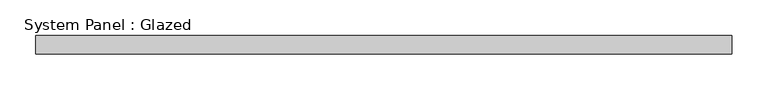
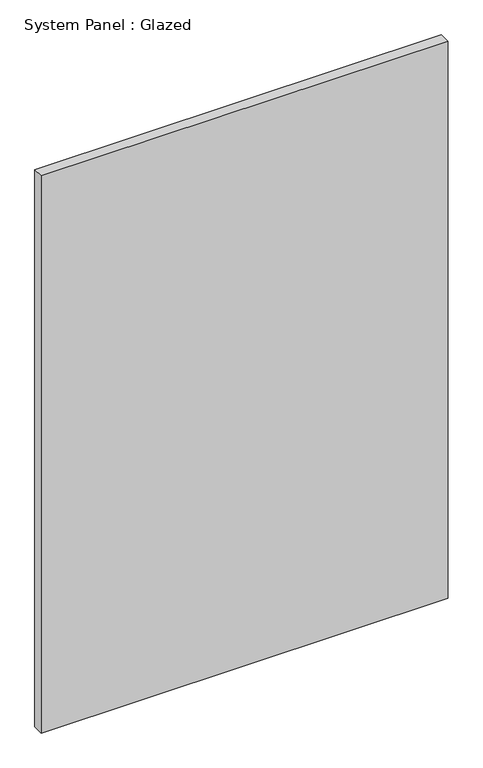
"""IFC4 building model written with IfcOpenShell, lengths in millimetres: plate geometry, System Panel : Glazed."""

from ifc_helpers import new_model, si_unit, origin, origin_with_axes, place, context, project, spatial, polyline, outline, extrude, source, transform, mapped, element, save


def system_panel_glazed_e1e0096c(model_context):
    return source(origin(), model_context, "Body", "SweptSolid", [
        extrude(outline(polyline([(485.775, 19.05), (-485.775, 19.05), (-485.775, 44.45), (485.775, 44.45), (485.775, 19.05)])), origin_with_axes(), (0.0, 0.0, 1.0), 1406.247479),
    ])


if __name__ == "__main__":
    model = new_model("IFC4")
    model_context = context("Model", 3, world=origin())
    ifc_project = project(units=[si_unit("LENGTHUNIT", "METRE", prefix="MILLI")], contexts=[model_context])
    site = spatial("IfcSite", under=ifc_project)
    building = spatial("IfcBuilding", under=site)
    placement = place(None, origin())
    system_panel_glazed_shape = system_panel_glazed_e1e0096c(model_context)
    element("IfcPlate", 1, ObjectType="System Panel : Glazed", at=placement, inside=building, context=model_context, shape_type="MappedRepresentation", body=[
        mapped(system_panel_glazed_shape, transform((0.0, 0.0, 0.0), x_axis=(1.0, 0.0, 0.0), y_axis=(0.0, 1.0, 0.0), z_axis=(0.0, 0.0, 1.0))),
    ])
    save(model, "model.ifc")

# Revit data of these elements
# Type "System Panel : Glazed"
#   Construction Type Id = "GSP4R"
#   Analytic Construction = "1/8 in Pilkington single glazing"
#   Visual Light Transmittance = 0.9
#   Solar Heat Gain Coefficient = 0.86
#   Heat Transfer Coefficient (U) = 1.18115 BTU/(h·ft²·°F)
#   Define Thermal Properties by = 1
# Element 1 (IfcPlate, "System Panel : Glazed")
#   Materials on its faces: "Glass"
# Materials
#   "Glass": class "Glass", colour RGB 0 128 192, transparency 0.75, Description = "Soda Lime Glass", Cost = 0
